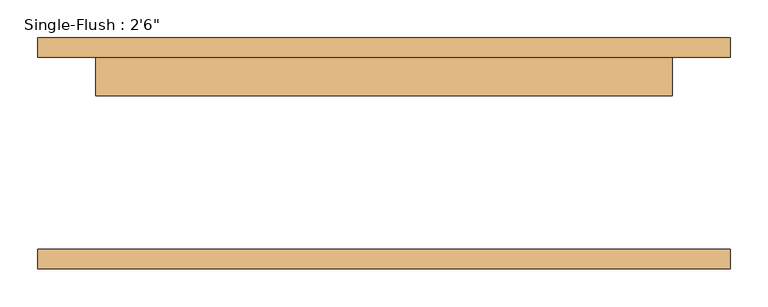
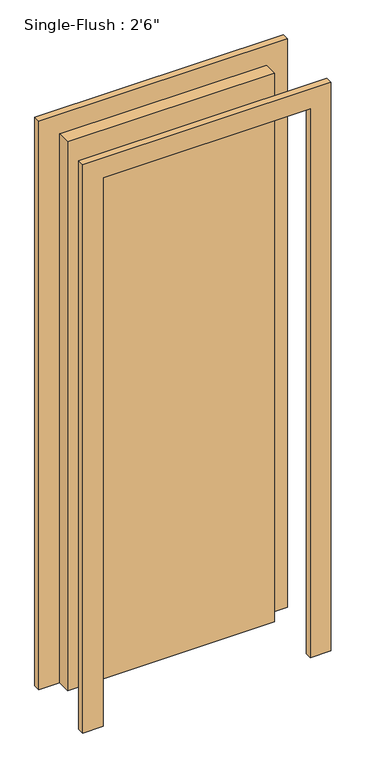
"""IFC4 building model written with IfcOpenShell, lengths in millimetres: door geometry."""

from ifc_helpers import new_model, si_unit, frame, origin, origin_with_axes, place, context, project, spatial, polyline, outline, extrude, source, transform, mapped, element, save


def door_bfeef022(model_context):
    return source(origin(), model_context, "Body", "SweptSolid", [
        extrude(outline(polyline([(2209.8, -457.2), (0.0, -457.2), (0.0, -381.0), (2133.6, -381.0), (2133.6, 381.0), (0.0, 381.0), (0.0, 457.2), (2209.8, 457.2), (2209.8, -457.2)])), frame((0.0, 127.0, 0.0), z_axis=(0.0, 1.0, 0.0), x_axis=(0.0, 0.0, 1.0)), (0.0, 0.0, 1.0), 25.4),
        extrude(outline(polyline([(2209.8, 457.2), (2209.8, -457.2), (0.0, -457.2), (0.0, -381.0), (2133.6, -381.0), (2133.6, 381.0), (0.0, 381.0), (0.0, 457.2), (2209.8, 457.2)])), frame((0.0, -152.4, 0.0), z_axis=(0.0, 1.0, 0.0), x_axis=(0.0, 0.0, 1.0)), (0.0, 0.0, 1.0), 25.4),
        extrude(outline(polyline([(381.0, 76.2), (-381.0, 76.2), (-381.0, 127.0), (381.0, 127.0), (381.0, 76.2)])), origin_with_axes(), (0.0, 0.0, 1.0), 2133.6),
    ])


if __name__ == "__main__":
    model = new_model("IFC4")
    model_context = context("Model", 3, world=origin())
    ifc_project = project(units=[si_unit("LENGTHUNIT", "METRE", prefix="MILLI")], contexts=[model_context])
    site = spatial("IfcSite", under=ifc_project)
    building = spatial("IfcBuilding", under=site)
    placement = place(None, origin())
    door_shape = door_bfeef022(model_context)
    element("IfcDoor", 1, ObjectType="Single-Flush : 2'6\"", at=placement, inside=building, context=model_context, shape_type="MappedRepresentation", body=[
        mapped(door_shape, transform((0.0, 0.0, 0.0), x_axis=(1.0, 0.0, 0.0), y_axis=(0.0, 1.0, 0.0), z_axis=(0.0, 0.0, 1.0))),
    ])
    save(model, "model.ifc")

# Revit data of these elements
# Type "Single-Flush : 2'6\""
#   Type Mark = "12"
#   Construction Type Id = "MDOOR"
#   Assembly Code = "C1020"
#   Analytic Construction = "Metal"
#   Thickness = 0' - 2"
#   Heat Transfer Coefficient (U) = 0.651978 BTU/(h·ft²·°F)
#   Height = 7' - 0"
#   Trim Projection Ext = 0' - 1"
#   Trim Projection Int = 0' - 1"
#   Trim Width = 0' - 3"
#   Width = 2' - 6"
#   Define Thermal Properties by = 1
#   Door Material = Door - Panel
#   Frame Material = Door - Frame
#   Visual Light Transmittance = 0
#   Solar Heat Gain Coefficient = 0
#   Function = (empty or 0)
#   Wall Closure = (empty or 0)
# Element 1 (IfcDoor, "Single-Flush : 2'6\"")
#   Materials on its faces: "Door - Frame", "Door - Panel"
# Materials
#   "Door - Panel": class "Wood", colour RGB 210 159 95, transparency 0, Cost = 0
#   "Door - Frame": colour RGB 118 70 51, transparency 0, Cost = 0
